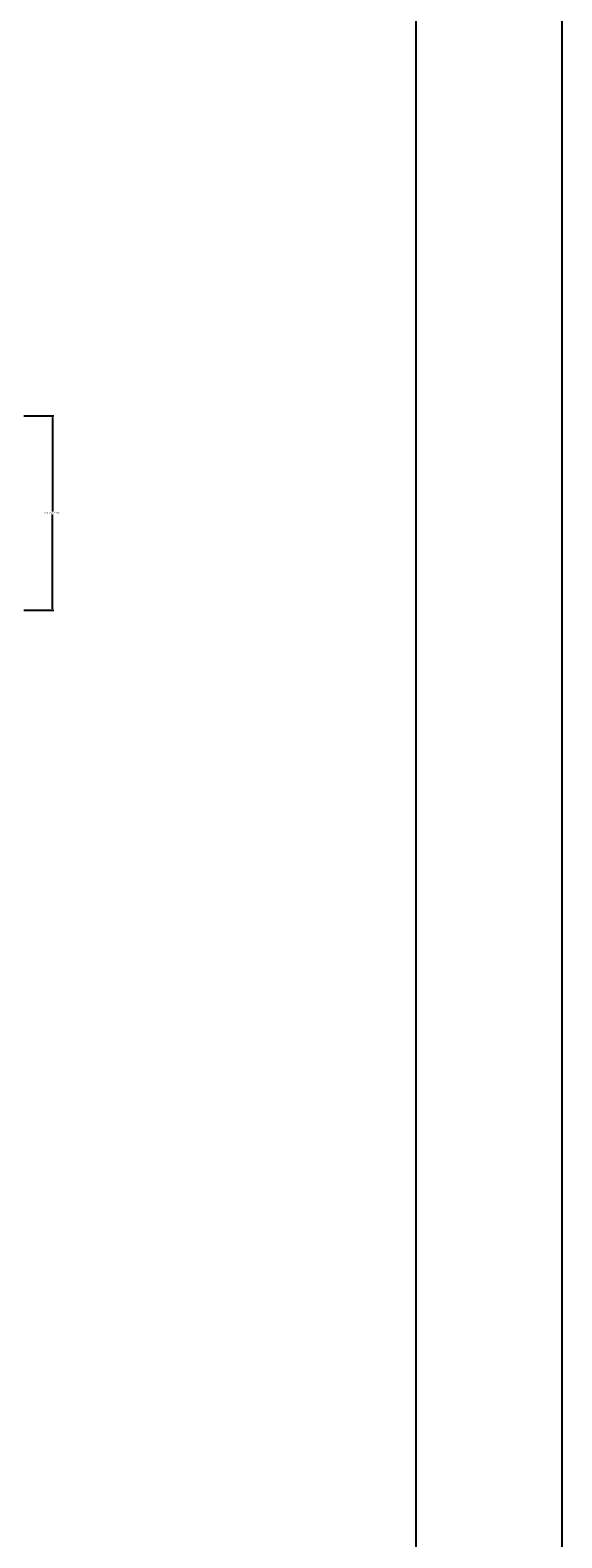
# Model space of a CAD drawing. Units: inches. Extents: x 1601 to 2297, y 1496 to 2631.
# Tile 50 of 57: x 2231 to 2297, y 2141 to 2327. Entities that reach past the tile are written whole.
import ezdxf

# ---------------------------------------------------------------- set-up
doc = ezdxf.new("R2010")
doc.units = ezdxf.units.IN
doc.layers.add('A-ANNO-DIMS', color=2, linetype='Continuous', lineweight=18)
doc.layers.add('A-ANNO-TTLB', color=7, linetype='Continuous', lineweight=25)
doc.styles.get("Standard").update_dxf_attribs({"font": 'arial.ttf'})
doc.dimstyles.get("Standard").update_dxf_attribs({"dimtxt": 0.18, "dimasz": 0.18, "dimexe": 0.18, "dimexo": 0.0625, "dimgap": 0.09, "dimtad": 0, "dimtih": 1, "dimtoh": 1, "dimdec": 4, "dimzin": 0, "dimdsep": 46, "dimtxsty": 'Standard', "dimcen": 0.09, "dimadec": 0, "dimazin": 0, "dimtfac": 1, "dimtdec": 4, "dimtofl": 0, "dimtmove": 0, "dimatfit": 3, "dimfxl": 1, "dimtolj": 1, "dimtzin": 0, "dimarcsym": 0})

# ---------------------------------------------------------------- blocks, each defined once
blk = doc.blocks.new('*D22')
at = {"layer": 'A-ANNO-DIMS', "color": 0, "lineweight": -2, "transparency": 16777216}
for p, q in [((2230.6, 2279.25), (2234.32, 2279.25)), ((2234.14, 2279.07), (2234.14, 2267.43)), ((2234.14, 2255.43), (2234.14, 2267.06)), ((2230.6, 2255.25), (2234.32, 2255.25))]:
    blk.add_line(p, q, dxfattribs=at)
at = {"layer": 'A-ANNO-DIMS', "color": 0, "transparency": 16777216}
for points in [[(2234.11, 2279.07), (2234.17, 2279.07), (2234.14, 2279.25)], [(2234.11, 2255.43), (2234.17, 2255.43), (2234.14, 2255.25)]]:
    blk.add_solid(points, dxfattribs=at)
at = {"layer": 'Defpoints', "color": 0, "transparency": 16777216}
for p in [(2230.54, 2279.25), (2234.14, 2279.25), (2230.54, 2255.25)]:
    blk.add_point(p, dxfattribs=at)
at = {"layer": 'A-ANNO-DIMS', "color": 0, "transparency": 16777216, "insert": (2234.14, 2267.25), "char_height": 0.18, "attachment_point": 5}
blk.add_mtext('\\A1;WINDOW 24 TYP.', dxfattribs=at)
blk = doc.blocks.new('*D29')
at = {"layer": 'A-ANNO-DIMS', "color": 0, "lineweight": -2, "transparency": 16777216}
for p, q in [((2230.6, 2532.33), (2279.27, 2532.33)), ((2279.09, 2532.15), (2279.09, 2084.01)), ((2279.09, 1635.51), (2279.09, 2083.64)), ((2230.6, 1635.33), (2279.27, 1635.33))]:
    blk.add_line(p, q, dxfattribs=at)
at = {"layer": 'A-ANNO-DIMS', "color": 0, "transparency": 16777216}
for points in [[(2279.06, 2532.15), (2279.12, 2532.15), (2279.09, 2532.33)], [(2279.06, 1635.51), (2279.12, 1635.51), (2279.09, 1635.33)]]:
    blk.add_solid(points, dxfattribs=at)
at = {"layer": 'Defpoints', "color": 0, "transparency": 16777216}
for p in [(2230.54, 2532.33), (2279.09, 2532.33), (2230.54, 1635.33)]:
    blk.add_point(p, dxfattribs=at)
at = {"layer": 'A-ANNO-DIMS', "color": 0, "transparency": 16777216, "insert": (2279.09, 2083.83), "char_height": 0.18, "attachment_point": 5}
blk.add_mtext('\\A1;897', dxfattribs=at)

msp = doc.modelspace()

# ---------------------------------------------------------------- linework, layer by layer
at = {"layer": 'A-ANNO-TTLB'}
msp.add_lwpolyline([(1600.5933, 2631.1477), (2297.129, 2631.1477), (2297.129, 1496.1026), (1600.5933, 1496.1026)], close=True, dxfattribs=at)

# ---------------------------------------------------------------- dimensions: what is measured, and where the dimension line sits
at = {"layer": 'A-ANNO-DIMS'}
dim = msp.add_linear_dim(base=(2279.0873, 2532.3254), p1=(2230.5373, 1635.3254), p2=(2230.5373, 2532.3254), angle=90, dimstyle='Standard', override={"dimdec": 0, "dimlfac": 1, "dimrnd": 0, "dimzin": 0, "dimdsep": 46, "dimlunit": 2}, dxfattribs=at)
dim.commit()
dim.dimension.update_dxf_attribs({"geometry": '*D29', "text_midpoint": (2279.0873, 2083.8254)})
dim = msp.add_linear_dim(base=(2234.1373, 2279.2475), p1=(2230.5373, 2255.2475), p2=(2230.5373, 2279.2475), angle=90, text='WINDOW <> TYP.', dimstyle='Standard', override={"dimdec": 0, "dimlfac": 1, "dimrnd": 0, "dimzin": 0, "dimdsep": 46, "dimlunit": 2}, dxfattribs=at)
dim.commit()
dim.dimension.update_dxf_attribs({"geometry": '*D22', "text_midpoint": (2234.1373, 2267.2475)})

doc.saveas('drawing.dxf')
